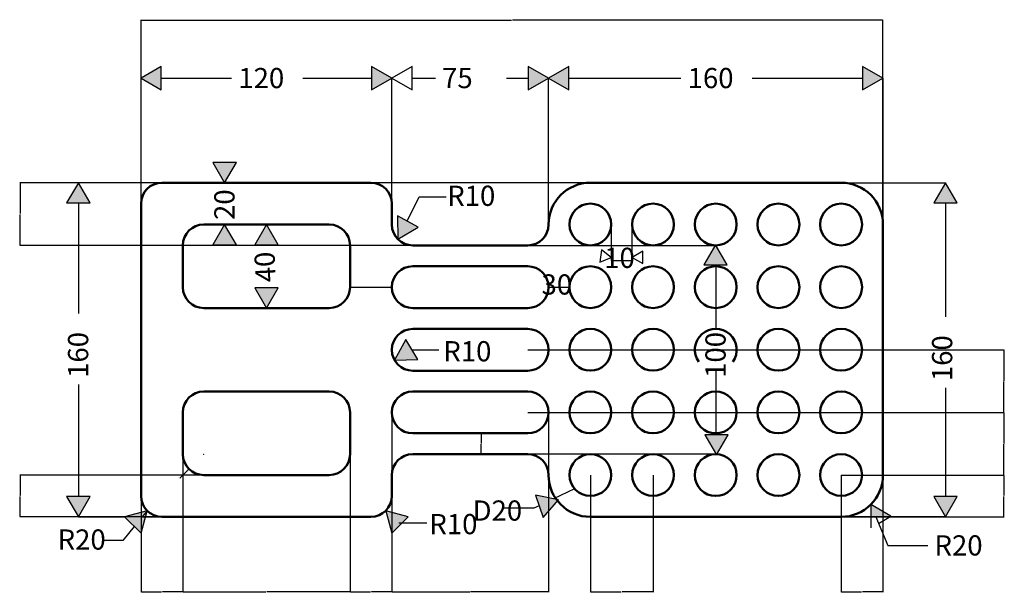
# Model space of a CAD drawing. Units: millimetres. Extents: x 384 to 855, y 1163 to 1437.
import ezdxf

# ---------------------------------------------------------------- set-up
doc = ezdxf.new("R2010")
doc.units = ezdxf.units.MM
for name, color, linetype, lineweight in [('M-DIMS', 2, 'Continuous', 25), ('M-HATC', 8, 'Continuous', 18), ('M-OUTL', 7, 'Continuous', 50), ('M-TEXT', 7, 'Continuous', 25)]:
    doc.layers.add(name, color=color, linetype=linetype, lineweight=lineweight)
doc.styles.get("Standard").update_dxf_attribs({"font": 'arial.ttf'})
doc.dimstyles.get("Standard").update_dxf_attribs({"dimtxt": 0.18, "dimasz": 0.18, "dimexe": 0.18, "dimexo": 0.0625, "dimgap": 0.09, "dimtad": 0, "dimtih": 1, "dimtoh": 1, "dimdec": 4, "dimzin": 0, "dimdsep": 46, "dimtxsty": 'Standard', "dimcen": 0.09, "dimadec": 0, "dimazin": 0, "dimtfac": 1, "dimtdec": 4, "dimtofl": 0, "dimtmove": 0, "dimatfit": 3, "dimfxl": 1, "dimtolj": 1, "dimtzin": 0, "dimarcsym": 0})

# ---------------------------------------------------------------- blocks, each defined once
blk = doc.blocks.new('HOLE-D20')
blk.add_circle((10, 10), 10)
blk = doc.blocks.new('OPENING-80X40-R10')
for p, q in [((10, 40), (70, 40)), ((0, 30), (0, 10)), ((80, 30), (80, 10)), ((10, 0), (70, 0))]:
    blk.add_line(p, q)
for centre, start, end in [((10, 30), 90, 180), ((70, 30), 0, 90), ((10, 10), 180, 270), ((70, 10), 270, 0)]:
    blk.add_arc(centre, 10, start, end)
blk = doc.blocks.new('SLOT-75X20-R10')
for p, q in [((10, 20), (65, 20)), ((10, 0), (65, 0))]:
    blk.add_line(p, q)
for centre, start, end in [((10, 10), 90, 270), ((65, 10), 270, 90)]:
    blk.add_arc(centre, 10, start, end)
blk = doc.blocks.new('DIM-ARROW-SMALL')
blk.add_lwpolyline([(0, 2.97), (5.15, 0), (5.15, 5.95)], close=True)
blk = doc.blocks.new('*D5')
at = {"layer": 'Defpoints', "color": 0, "transparency": 16777216}
for p in [(796.88, 1437.22), (441.88, 1349.32), (796.88, 1339.32)]:
    blk.add_point(p, dxfattribs=at)
at = {"layer": 'M-DIMS', "color": 0, "lineweight": -2, "transparency": 16777216}
for p, q in [((441.88, 1349.39), (441.88, 1437.4)), ((442.06, 1437.22), (619.09, 1437.22)), ((796.7, 1437.22), (619.67, 1437.22)), ((796.88, 1339.39), (796.88, 1437.4))]:
    blk.add_line(p, q, dxfattribs=at)
at = {"layer": 'M-DIMS', "color": 0, "transparency": 16777216}
for points in [[(442.06, 1437.25), (442.06, 1437.19), (441.88, 1437.22)], [(796.7, 1437.25), (796.7, 1437.19), (796.88, 1437.22)]]:
    blk.add_solid(points, dxfattribs=at)
at = {"layer": 'M-DIMS', "color": 0, "transparency": 16777216, "insert": (619.38, 1437.22), "char_height": 0.18, "attachment_point": 5}
blk.add_mtext('\\A1;355', dxfattribs=at)
blk = doc.blocks.new('*D6')
at = {"layer": 'Defpoints', "color": 0, "transparency": 16777216}
for p in [(461.88, 1229.32), (441.88, 1209.32), (461.88, 1163.36)]:
    blk.add_point(p, dxfattribs=at)
at = {"layer": 'M-DIMS', "color": 0, "lineweight": -2, "transparency": 16777216}
for p, q in [((461.88, 1229.26), (461.88, 1163.18)), ((441.88, 1209.26), (441.88, 1163.18)), ((442.06, 1163.36), (451.66, 1163.36)), ((461.7, 1163.36), (452.1, 1163.36))]:
    blk.add_line(p, q, dxfattribs=at)
at = {"layer": 'M-DIMS', "color": 0, "transparency": 16777216}
for points in [[(442.06, 1163.39), (442.06, 1163.33), (441.88, 1163.36)], [(461.7, 1163.39), (461.7, 1163.33), (461.88, 1163.36)]]:
    blk.add_solid(points, dxfattribs=at)
at = {"layer": 'M-DIMS', "color": 0, "transparency": 16777216, "insert": (451.88, 1163.36), "char_height": 0.18, "attachment_point": 5}
blk.add_mtext('\\A1;20', dxfattribs=at)
blk = doc.blocks.new('*D7')
at = {"layer": 'Defpoints', "color": 0, "transparency": 16777216}
for p in [(461.88, 1229.32), (541.88, 1229.32), (541.88, 1163.36)]:
    blk.add_point(p, dxfattribs=at)
at = {"layer": 'M-DIMS', "color": 0, "lineweight": -2, "transparency": 16777216}
for p, q in [((461.88, 1229.26), (461.88, 1163.18)), ((541.88, 1229.26), (541.88, 1163.18)), ((462.06, 1163.36), (501.66, 1163.36)), ((541.7, 1163.36), (502.1, 1163.36))]:
    blk.add_line(p, q, dxfattribs=at)
at = {"layer": 'M-DIMS', "color": 0, "transparency": 16777216}
for points in [[(462.06, 1163.39), (462.06, 1163.33), (461.88, 1163.36)], [(541.7, 1163.39), (541.7, 1163.33), (541.88, 1163.36)]]:
    blk.add_solid(points, dxfattribs=at)
at = {"layer": 'M-DIMS', "color": 0, "transparency": 16777216, "insert": (501.88, 1163.36), "char_height": 0.18, "attachment_point": 5}
blk.add_mtext('\\A1;80', dxfattribs=at)
blk = doc.blocks.new('*D8')
at = {"layer": 'Defpoints', "color": 0, "transparency": 16777216}
for p in [(561.88, 1249.32), (541.88, 1229.32), (561.88, 1163.36)]:
    blk.add_point(p, dxfattribs=at)
at = {"layer": 'M-DIMS', "color": 0, "lineweight": -2, "transparency": 16777216}
for p, q in [((561.88, 1249.26), (561.88, 1163.18)), ((541.88, 1229.26), (541.88, 1163.18)), ((542.06, 1163.36), (551.66, 1163.36)), ((561.7, 1163.36), (552.1, 1163.36))]:
    blk.add_line(p, q, dxfattribs=at)
at = {"layer": 'M-DIMS', "color": 0, "transparency": 16777216}
for points in [[(542.06, 1163.39), (542.06, 1163.33), (541.88, 1163.36)], [(561.7, 1163.39), (561.7, 1163.33), (561.88, 1163.36)]]:
    blk.add_solid(points, dxfattribs=at)
at = {"layer": 'M-DIMS', "color": 0, "transparency": 16777216, "insert": (551.88, 1163.36), "char_height": 0.18, "attachment_point": 5}
blk.add_mtext('\\A1;20', dxfattribs=at)
blk = doc.blocks.new('*D9')
at = {"layer": 'Defpoints', "color": 0, "transparency": 16777216}
for p in [(561.88, 1249.32), (636.88, 1249.32), (636.88, 1163.36)]:
    blk.add_point(p, dxfattribs=at)
at = {"layer": 'M-DIMS', "color": 0, "lineweight": -2, "transparency": 16777216}
for p, q in [((561.88, 1249.26), (561.88, 1163.18)), ((636.88, 1249.26), (636.88, 1163.18)), ((562.06, 1163.36), (599.16, 1163.36)), ((636.7, 1163.36), (599.6, 1163.36))]:
    blk.add_line(p, q, dxfattribs=at)
at = {"layer": 'M-DIMS', "color": 0, "transparency": 16777216}
for points in [[(562.06, 1163.39), (562.06, 1163.33), (561.88, 1163.36)], [(636.7, 1163.39), (636.7, 1163.33), (636.88, 1163.36)]]:
    blk.add_solid(points, dxfattribs=at)
at = {"layer": 'M-DIMS', "color": 0, "transparency": 16777216, "insert": (599.38, 1163.36), "char_height": 0.18, "attachment_point": 5}
blk.add_mtext('\\A1;75', dxfattribs=at)
blk = doc.blocks.new('*D10')
at = {"layer": 'Defpoints', "color": 0, "transparency": 16777216}
for p in [(383.98, 1219.32), (471.88, 1219.32), (451.88, 1199.32)]:
    blk.add_point(p, dxfattribs=at)
at = {"layer": 'M-DIMS', "color": 0, "lineweight": -2, "transparency": 16777216}
for p, q in [((471.82, 1219.32), (383.8, 1219.32)), ((383.98, 1219.14), (383.98, 1209.51)), ((383.98, 1199.5), (383.98, 1209.14)), ((451.82, 1199.32), (383.8, 1199.32))]:
    blk.add_line(p, q, dxfattribs=at)
at = {"layer": 'M-DIMS', "color": 0, "transparency": 16777216}
for points in [[(383.95, 1219.14), (384.01, 1219.14), (383.98, 1219.32)], [(383.95, 1199.5), (384.01, 1199.5), (383.98, 1199.32)]]:
    blk.add_solid(points, dxfattribs=at)
at = {"layer": 'M-DIMS', "color": 0, "transparency": 16777216, "insert": (383.98, 1209.32), "char_height": 0.18, "attachment_point": 5}
blk.add_mtext('\\A1;20', dxfattribs=at)
blk = doc.blocks.new('*D11')
at = {"layer": 'Defpoints', "color": 0, "transparency": 16777216}
for p in [(383.98, 1359.32), (656.88, 1359.32), (626.88, 1329.32)]:
    blk.add_point(p, dxfattribs=at)
at = {"layer": 'M-DIMS', "color": 0, "lineweight": -2, "transparency": 16777216}
for p, q in [((656.82, 1359.32), (383.8, 1359.32)), ((383.98, 1359.14), (383.98, 1344.51)), ((383.98, 1329.5), (383.98, 1344.14)), ((626.82, 1329.32), (383.8, 1329.32))]:
    blk.add_line(p, q, dxfattribs=at)
at = {"layer": 'M-DIMS', "color": 0, "transparency": 16777216}
for points in [[(383.95, 1359.14), (384.01, 1359.14), (383.98, 1359.32)], [(383.95, 1329.5), (384.01, 1329.5), (383.98, 1329.32)]]:
    blk.add_solid(points, dxfattribs=at)
at = {"layer": 'M-DIMS', "color": 0, "transparency": 16777216, "insert": (383.98, 1344.32), "char_height": 0.18, "attachment_point": 5}
blk.add_mtext('\\A1;30', dxfattribs=at)
blk = doc.blocks.new('*D12')
at = {"layer": 'Defpoints', "color": 0, "transparency": 16777216}
for p in [(626.88, 1279.32), (854.78, 1279.32), (626.88, 1249.32)]:
    blk.add_point(p, dxfattribs=at)
at = {"layer": 'M-DIMS', "color": 0, "lineweight": -2, "transparency": 16777216}
for p, q in [((626.94, 1279.32), (854.96, 1279.32)), ((854.78, 1279.14), (854.78, 1264.51)), ((854.78, 1249.5), (854.78, 1264.14)), ((626.94, 1249.32), (854.96, 1249.32))]:
    blk.add_line(p, q, dxfattribs=at)
at = {"layer": 'M-DIMS', "color": 0, "transparency": 16777216}
for points in [[(854.75, 1279.14), (854.81, 1279.14), (854.78, 1279.32)], [(854.75, 1249.5), (854.81, 1249.5), (854.78, 1249.32)]]:
    blk.add_solid(points, dxfattribs=at)
at = {"layer": 'M-DIMS', "color": 0, "transparency": 16777216, "insert": (854.78, 1264.32), "char_height": 0.18, "attachment_point": 5}
blk.add_mtext('\\A1;30', dxfattribs=at)
blk = doc.blocks.new('*D13')
at = {"layer": 'Defpoints', "color": 0, "transparency": 16777216}
for p in [(604.58, 1239.32), (626.88, 1239.32), (626.88, 1229.32)]:
    blk.add_point(p, dxfattribs=at)
at = {"layer": 'M-DIMS', "color": 0, "lineweight": -2, "transparency": 16777216}
for p, q in [((626.82, 1239.32), (604.4, 1239.32)), ((604.58, 1239.14), (604.58, 1234.51)), ((604.58, 1229.5), (604.58, 1234.14)), ((626.82, 1229.32), (604.4, 1229.32))]:
    blk.add_line(p, q, dxfattribs=at)
at = {"layer": 'M-DIMS', "color": 0, "transparency": 16777216}
for points in [[(604.55, 1239.14), (604.61, 1239.14), (604.58, 1239.32)], [(604.55, 1229.5), (604.61, 1229.5), (604.58, 1229.32)]]:
    blk.add_solid(points, dxfattribs=at)
at = {"layer": 'M-DIMS', "color": 0, "transparency": 16777216, "insert": (604.58, 1234.32), "char_height": 0.18, "attachment_point": 5}
blk.add_mtext('\\A1;10', dxfattribs=at)
blk = doc.blocks.new('*D14')
at = {"layer": 'Defpoints', "color": 0, "transparency": 16777216}
for p in [(656.88, 1219.32), (686.88, 1219.32), (686.88, 1163.36)]:
    blk.add_point(p, dxfattribs=at)
at = {"layer": 'M-DIMS', "color": 0, "lineweight": -2, "transparency": 16777216}
for p, q in [((656.88, 1219.26), (656.88, 1163.18)), ((686.88, 1219.26), (686.88, 1163.18)), ((657.06, 1163.36), (671.66, 1163.36)), ((686.7, 1163.36), (672.1, 1163.36))]:
    blk.add_line(p, q, dxfattribs=at)
at = {"layer": 'M-DIMS', "color": 0, "transparency": 16777216}
for points in [[(657.06, 1163.39), (657.06, 1163.33), (656.88, 1163.36)], [(686.7, 1163.39), (686.7, 1163.33), (686.88, 1163.36)]]:
    blk.add_solid(points, dxfattribs=at)
at = {"layer": 'M-DIMS', "color": 0, "transparency": 16777216, "insert": (671.88, 1163.36), "char_height": 0.18, "attachment_point": 5}
blk.add_mtext('\\A1;30', dxfattribs=at)
blk = doc.blocks.new('*D15')
at = {"layer": 'Defpoints', "color": 0, "transparency": 16777216}
for p in [(776.88, 1249.32), (854.78, 1249.32), (776.88, 1219.32)]:
    blk.add_point(p, dxfattribs=at)
at = {"layer": 'M-DIMS', "color": 0, "lineweight": -2, "transparency": 16777216}
for p, q in [((776.94, 1249.32), (854.96, 1249.32)), ((854.78, 1249.14), (854.78, 1234.51)), ((854.78, 1219.5), (854.78, 1234.14)), ((776.94, 1219.32), (854.96, 1219.32))]:
    blk.add_line(p, q, dxfattribs=at)
at = {"layer": 'M-DIMS', "color": 0, "transparency": 16777216}
for points in [[(854.75, 1249.14), (854.81, 1249.14), (854.78, 1249.32)], [(854.75, 1219.5), (854.81, 1219.5), (854.78, 1219.32)]]:
    blk.add_solid(points, dxfattribs=at)
at = {"layer": 'M-DIMS', "color": 0, "transparency": 16777216, "insert": (854.78, 1234.32), "char_height": 0.18, "attachment_point": 5}
blk.add_mtext('\\A1;30', dxfattribs=at)
blk = doc.blocks.new('*D16')
at = {"layer": 'Defpoints', "color": 0, "transparency": 16777216}
for p in [(776.88, 1219.32), (796.88, 1219.32), (796.88, 1163.36)]:
    blk.add_point(p, dxfattribs=at)
at = {"layer": 'M-DIMS', "color": 0, "lineweight": -2, "transparency": 16777216}
for p, q in [((776.88, 1219.26), (776.88, 1163.18)), ((796.88, 1219.26), (796.88, 1163.18)), ((777.06, 1163.36), (786.66, 1163.36)), ((796.7, 1163.36), (787.1, 1163.36))]:
    blk.add_line(p, q, dxfattribs=at)
at = {"layer": 'M-DIMS', "color": 0, "transparency": 16777216}
for points in [[(777.06, 1163.39), (777.06, 1163.33), (776.88, 1163.36)], [(796.7, 1163.39), (796.7, 1163.33), (796.88, 1163.36)]]:
    blk.add_solid(points, dxfattribs=at)
at = {"layer": 'M-DIMS', "color": 0, "transparency": 16777216, "insert": (786.88, 1163.36), "char_height": 0.18, "attachment_point": 5}
blk.add_mtext('\\A1;20', dxfattribs=at)
blk = doc.blocks.new('*D17')
at = {"layer": 'Defpoints', "color": 0, "transparency": 16777216}
for p in [(776.88, 1219.32), (854.78, 1219.32), (776.88, 1199.32)]:
    blk.add_point(p, dxfattribs=at)
at = {"layer": 'M-DIMS', "color": 0, "lineweight": -2, "transparency": 16777216}
for p, q in [((776.94, 1219.32), (854.96, 1219.32)), ((854.78, 1219.14), (854.78, 1209.51)), ((854.78, 1199.5), (854.78, 1209.14)), ((776.94, 1199.32), (854.96, 1199.32))]:
    blk.add_line(p, q, dxfattribs=at)
at = {"layer": 'M-DIMS', "color": 0, "transparency": 16777216}
for points in [[(854.75, 1219.14), (854.81, 1219.14), (854.78, 1219.32)], [(854.75, 1199.5), (854.81, 1199.5), (854.78, 1199.32)]]:
    blk.add_solid(points, dxfattribs=at)
at = {"layer": 'M-DIMS', "color": 0, "transparency": 16777216, "insert": (854.78, 1209.32), "char_height": 0.18, "attachment_point": 5}
blk.add_mtext('\\A1;20', dxfattribs=at)
blk = doc.blocks.new('*D18')
at = {"layer": 'Defpoints', "color": 0, "transparency": 16777216}
for p in [(471.88, 1229.32), (464.81, 1222.25)]:
    blk.add_point(p, dxfattribs=at)
at = {"layer": 'M-DIMS', "color": 0, "lineweight": -2, "transparency": 16777216}
for p, q in [((471.79, 1229.32), (471.97, 1229.32)), ((471.88, 1229.23), (471.88, 1229.41)), ((460.57, 1218.01), (464.68, 1222.12)), ((460.39, 1218.01), (460.57, 1218.01))]:
    blk.add_line(p, q, dxfattribs=at)
at = {"layer": 'M-DIMS', "color": 0, "transparency": 16777216}
blk.add_solid([(464.66, 1222.15), (464.71, 1222.1), (464.81, 1222.25)], dxfattribs=at)
at = {"layer": 'M-DIMS', "color": 0, "transparency": 16777216, "insert": (459.89, 1218.01), "char_height": 0.18, "attachment_point": 5}
blk.add_mtext('\\A1;8X R10', dxfattribs=at)

msp = doc.modelspace()

# ---------------------------------------------------------------- hatches: boundary and pattern name
at = {"layer": 'M-HATC'}
h = msp.add_hatch(color=256, dxfattribs=at)
h.dxf.hatch_style = 1
h.paths.add_polyline_path([(411.88, 1359.32), (406.28, 1349.63), (417.48, 1349.63)])
h.paths.add_polyline_path([(417.48, 1209.02), (406.28, 1209.02), (411.88, 1199.32)])
h.paths.add_polyline_path([(444.03, 1199.32), (442.41, 1199.32), (444.81, 1202.25), (434, 1199.36), (441.91, 1191.44)])
h.paths.add_polyline_path([(487.48, 1369.02), (476.28, 1369.02), (481.88, 1359.32)])
h.paths.add_polyline_path([(481.88, 1339.32), (476.28, 1329.63), (487.48, 1329.63)])
h.paths.add_polyline_path([(501.88, 1339.32), (496.28, 1329.63), (507.48, 1329.63)])
h.paths.add_polyline_path([(507.48, 1309.02), (496.28, 1309.02), (501.88, 1299.32)])
h.paths.add_polyline_path([(451.58, 1414.92), (441.88, 1409.32), (451.58, 1403.73)])
h.paths.add_polyline_path([(552.18, 1414.92), (552.18, 1403.73), (561.88, 1409.32)])
h.paths.add_polyline_path([(574.42, 1338.01), (564.63, 1343.45), (564.81, 1332.25)])
h.paths.add_polyline_path([(636.88, 1409.32), (627.18, 1414.92), (627.18, 1403.73)])
h.paths.add_polyline_path([(646.58, 1414.92), (636.88, 1409.32), (646.58, 1403.73)])
h.paths.add_polyline_path([(787.18, 1414.92), (787.18, 1403.73), (796.88, 1409.32)])
h.paths.add_polyline_path([(826.88, 1359.32), (821.28, 1349.63), (832.48, 1349.63)])
h.paths.add_polyline_path([(832.48, 1209.02), (821.28, 1209.02), (826.88, 1199.32)])
h.paths.add_polyline_path([(791.02, 1205.18), (791.02, 1199.32), (800.27, 1199.32), (800.72, 1199.58)])
h.paths.add_polyline_path([(641.17, 1206.95, -0.012246), (640.58, 1207.73), (630.67, 1209.63), (634.35, 1199.05)])
h.paths.add_polyline_path([(558.95, 1202.25), (561.85, 1191.44), (569.77, 1199.36)])
h.paths.add_polyline_path([(568.51, 1284.25), (563.17, 1274.41), (574.36, 1274.71)])
h.paths.add_polyline_path([(716.98, 1329.32), (716.6, 1329.32), (711.19, 1319.96), (722.39, 1319.96)])
h.paths.add_polyline_path([(726.88, 1219.32, -1), (706.88, 1219.32, -0.414214), (716.88, 1229.32), (716.88, 1229.59), (711.64, 1238.66), (716.88, 1238.66), (716.88, 1239.32, -0.414214), (706.88, 1249.32, -1), (726.88, 1249.32, -0.414214), (716.88, 1239.32), (716.88, 1238.66), (722.84, 1238.66), (717.44, 1229.31, -0.397898)])
h.paths.add_polyline_path([(726.88, 1219.32, 0.397898), (717.44, 1229.31), (717.24, 1228.96), (717.03, 1229.32, 0.418706), (706.88, 1219.32, 1)])
h.paths.add_polyline_path([(716.88, 1259.32, 0.414214), (706.88, 1249.32, 0.414214), (716.88, 1239.32)], flags=17)
h.paths.add_polyline_path([(716.88, 1259.32), (716.88, 1239.32, 0.414214), (726.88, 1249.32, 0.414214)], flags=17)

# ---------------------------------------------------------------- linework, layer by layer
at = {"layer": 'M-DIMS'}
for p, q in [((441.88, 1349.32), (441.88, 1409.32)), ((451.58, 1409.32), (485.21, 1409.32)), ((519.27, 1409.32), (552.18, 1409.32)), ((561.88, 1339.32), (561.88, 1409.32)), ((571.58, 1409.32), (582.71, 1409.32)), ((616.77, 1409.32), (627.18, 1409.32)), ((636.88, 1339.32), (636.88, 1409.32)), ((646.58, 1409.32), (700.21, 1409.32)), ((734.27, 1409.32), (787.18, 1409.32)), ((796.88, 1409.32), (796.88, 1339.32)), ((451.88, 1359.32), (411.88, 1359.32)), ((501.88, 1359.32), (461.88, 1359.32)), ((776.88, 1359.32), (796.88, 1359.32)), ((796.88, 1359.32), (826.88, 1359.32)), ((569.15, 1340.93), (574.95, 1352.5)), ((574.95, 1352.5), (587.94, 1352.5)), ((411.88, 1349.63), (411.88, 1296.71)), ((826.88, 1349.63), (826.88, 1295.15)), ((666.88, 1339.32), (666.88, 1322.08)), ((676.88, 1322.08), (676.88, 1339.32)), ((626.88, 1329.32), (716.88, 1329.32)), ((666.88, 1322.08), (676.88, 1322.08)), ((716.88, 1319.96), (716.88, 1289.32)), ((541.88, 1309.32), (561.88, 1309.32)), ((636.88, 1309.32), (646.88, 1309.32)), ((571.62, 1279.18), (571.88, 1279.32)), ((571.88, 1279.32), (584.29, 1279.32)), ((716.88, 1269.32), (716.88, 1238.66)), ((411.88, 1262.66), (411.88, 1209.02)), ((826.88, 1261.1), (826.88, 1209.02)), ((716.88, 1229.32), (626.88, 1229.32)), ((716.88, 1229.59), (716.88, 1229.32)), ((649.32, 1212.78), (639.31, 1207.97)), ((444.81, 1202.25), (442.41, 1199.32)), ((629.79, 1203.41), (615.58, 1203.41)), ((632.4, 1204.66), (629.79, 1203.41)), ((411.88, 1199.32), (434.03, 1199.32)), ((442.41, 1199.32), (451.88, 1199.32)), ((826.88, 1199.32), (776.88, 1199.32)), ((793.49, 1199.32), (799.23, 1185.66)), ((438.63, 1194.72), (433.12, 1188.01)), ((565.2, 1196.51), (578.6, 1196.51)), ((433.12, 1188.01), (423.38, 1188.01)), ((799.23, 1185.66), (818.32, 1185.66))]:
    msp.add_line(p, q, dxfattribs=at)
for points in [[(441.88, 1409.32), (451.58, 1403.73), (451.58, 1414.92)], [(561.88, 1409.32), (552.18, 1414.92), (552.18, 1403.73)], [(561.88, 1409.32), (571.58, 1403.73), (571.58, 1414.92)], [(636.88, 1409.32), (627.18, 1414.92), (627.18, 1403.73)], [(636.88, 1409.32), (646.58, 1403.73), (646.58, 1414.92)], [(796.88, 1409.32), (787.18, 1414.92), (787.18, 1403.73)], [(481.88, 1359.32), (487.48, 1369.02), (476.28, 1369.02)], [(411.88, 1359.32), (406.28, 1349.63), (417.48, 1349.63)], [(826.88, 1359.32), (821.28, 1349.63), (832.48, 1349.63)], [(564.63, 1343.45), (564.81, 1332.25), (574.42, 1338.01)], [(481.88, 1339.32), (476.28, 1329.63), (487.48, 1329.63)], [(501.88, 1339.32), (496.28, 1329.63), (507.48, 1329.63)], [(716.79, 1329.66), (711.19, 1319.96), (722.39, 1319.96)], [(501.88, 1299.32), (507.48, 1309.02), (496.28, 1309.02)], [(568.51, 1284.25), (563.17, 1274.41), (574.36, 1274.71)], [(717.24, 1228.96), (722.84, 1238.66), (711.64, 1238.66)], [(411.88, 1199.32), (417.48, 1209.02), (406.28, 1209.02)], [(630.67, 1209.63), (634.35, 1199.05), (641.67, 1207.52)], [(826.88, 1199.32), (832.48, 1209.02), (821.28, 1209.02)], [(444.81, 1202.25), (434, 1199.36), (441.91, 1191.44)], [(558.95, 1202.25), (561.85, 1191.44), (569.77, 1199.36)]]:
    msp.add_lwpolyline(points, close=True, dxfattribs=at)
msp.add_lwpolyline([(794.81, 1196.17), (800.72, 1199.58), (791.02, 1205.18), (791.02, 1193.99)], dxfattribs=at)
at = {"layer": 'M-OUTL'}
for p, q in [((551.88, 1359.32), (451.88, 1359.32)), ((656.88, 1359.32), (776.88, 1359.32)), ((441.88, 1209.32), (441.88, 1349.32)), ((561.88, 1339.32), (561.88, 1349.32)), ((796.88, 1339.32), (796.88, 1219.32)), ((571.88, 1329.32), (626.88, 1329.32)), ((571.88, 1229.32), (626.88, 1229.32)), ((561.88, 1209.32), (561.88, 1219.32)), ((451.88, 1199.32), (551.88, 1199.32)), ((656.88, 1199.32), (776.88, 1199.32))]:
    msp.add_line(p, q, dxfattribs=at)
for centre in [(716.88, 1249.32), (716.88, 1219.32)]:
    msp.add_circle(centre, 10, dxfattribs=at)
for centre, radius, start, end in [((451.88, 1349.32), 10, 90, 180), ((551.88, 1349.32), 10, 0, 90), ((656.88, 1339.32), 20, 90, 180), ((776.88, 1339.32), 20, 0, 90), ((571.88, 1339.32), 10, 180, 270), ((626.88, 1339.32), 10, 270, 0), ((716.88, 1279.32), 10, 324.5283, 215.1776), ((571.88, 1219.32), 10, 90, 180), ((626.88, 1219.32), 10, 0, 90), ((656.88, 1219.32), 20, 180, 270), ((776.88, 1219.32), 20, 270, 0), ((451.88, 1209.32), 10, 180, 270), ((551.88, 1209.32), 10, 270, 0)]:
    msp.add_arc(centre, radius, start, end, dxfattribs=at)

# ---------------------------------------------------------------- block references
at = {"layer": 'M-DIMS', "rotation": 171.8056456691831}
msp.add_blockref('DIM-ARROW-SMALL', (667.31, 1326.51), dxfattribs=at)
at = {"layer": 'M-DIMS'}
msp.add_blockref('DIM-ARROW-SMALL', (676.88, 1320.59), dxfattribs=at)
at = {"layer": 'M-OUTL'}
for name, p in [('HOLE-D20', (646.88, 1329.33)), ('HOLE-D20', (676.88, 1329.33)), ('HOLE-D20', (706.88, 1329.33)), ('HOLE-D20', (736.88, 1329.33)), ('HOLE-D20', (766.88, 1329.33)), ('OPENING-80X40-R10', (461.88, 1299.33)), ('SLOT-75X20-R10', (561.88, 1299.33)), ('HOLE-D20', (646.88, 1299.33)), ('HOLE-D20', (676.88, 1299.33)), ('HOLE-D20', (706.88, 1299.33)), ('HOLE-D20', (736.88, 1299.33)), ('HOLE-D20', (766.88, 1299.33)), ('HOLE-D20', (646.88, 1269.33)), ('HOLE-D20', (676.88, 1269.33)), ('HOLE-D20', (736.88, 1269.33)), ('HOLE-D20', (766.88, 1269.33)), ('OPENING-80X40-R10', (461.88, 1219.33)), ('HOLE-D20', (646.88, 1239.33)), ('HOLE-D20', (676.88, 1239.33)), ('HOLE-D20', (736.88, 1239.33)), ('HOLE-D20', (766.88, 1239.33)), ('HOLE-D20', (646.88, 1209.33)), ('HOLE-D20', (676.88, 1209.33)), ('HOLE-D20', (736.88, 1209.33)), ('HOLE-D20', (766.88, 1209.33))]:
    msp.add_blockref(name, p, dxfattribs=at)
at = {"layer": 'M-OUTL', "rotation": 180}
for p in [(636.88, 1289.32), (636.88, 1259.32)]:
    msp.add_blockref('SLOT-75X20-R10', p, dxfattribs=at)

# ---------------------------------------------------------------- texts
at = {"layer": 'M-TEXT', "char_height": 9.668, "attachment_point": 1}
for s, insert in [('120', (488.43, 1414.28)), ('75', (585.93, 1414.28)), ('160', (703.43, 1414.28)), ('R10', (588.37, 1357.9)), ('10', (663.51, 1328.19)), ('30', (633.51, 1315.43)), ('R10', (586.5, 1283.46)), ('D20', (600.53, 1207.18)), ('R10', (579.83, 1200.69)), ('R20', (401.95, 1193.3)), ('R20', (821.55, 1190.48))]:
    msp.add_mtext_dynamic_manual_height_columns(s, width=27.6087, gutter_width=48.34, heights=[0], dxfattribs=dict(at, insert=insert))
for s, insert, rotation in [('20', (476.93, 1341.5), 90), ('40', (496.79, 1311.41), 92.964), ('160', (406.93, 1265.88), 90), ('100', (711.93, 1265.88), 90), ('160', (820.37, 1264.32), 90)]:
    msp.add_mtext_dynamic_manual_height_columns(s, width=27.6087, gutter_width=48.34, heights=[0], dxfattribs=dict(at, insert=insert, rotation=rotation))

# ---------------------------------------------------------------- dimensions: what is measured, and where the dimension line sits
at = {"layer": 'M-DIMS'}
for base, p1, p2, picture, middle in [((796.88, 1437.22), (441.88, 1349.32), (796.88, 1339.32), '*D5', (619.38, 1437.22)), ((561.88, 1163.36), (541.88, 1229.32), (561.88, 1249.32), '*D8', (551.88, 1163.36)), ((636.88, 1163.36), (561.88, 1249.32), (636.88, 1249.32), '*D9', (599.38, 1163.36)), ((461.88, 1163.36), (441.88, 1209.32), (461.88, 1229.32), '*D6', (451.88, 1163.36)), ((541.88, 1163.36), (461.88, 1229.32), (541.88, 1229.32), '*D7', (501.88, 1163.36)), ((686.88, 1163.36), (656.88, 1219.32), (686.88, 1219.32), '*D14', (671.88, 1163.36)), ((796.88, 1163.36), (776.88, 1219.32), (796.88, 1219.32), '*D16', (786.88, 1163.36))]:
    dim = msp.add_linear_dim(base=base, p1=p1, p2=p2, dimstyle='Standard', override={"dimdec": 0, "dimlfac": 1, "dimrnd": 0, "dimzin": 0, "dimdsep": 46, "dimlunit": 2}, dxfattribs=at)
    dim.commit()
    dim.dimension.update_dxf_attribs({"geometry": picture, "text_midpoint": middle})
for base, p1, p2, picture, middle in [((383.98, 1359.32), (626.88, 1329.32), (656.88, 1359.32), '*D11', (383.98, 1344.32)), ((854.78, 1279.32), (626.88, 1249.32), (626.88, 1279.32), '*D12', (854.78, 1264.32)), ((854.78, 1249.32), (776.88, 1219.32), (776.88, 1249.32), '*D15', (854.78, 1234.32)), ((604.58, 1239.32), (626.88, 1229.32), (626.88, 1239.32), '*D13', (604.58, 1234.32)), ((383.98, 1219.32), (451.88, 1199.32), (471.88, 1219.32), '*D10', (383.98, 1209.32)), ((854.78, 1219.32), (776.88, 1199.32), (776.88, 1219.32), '*D17', (854.78, 1209.32))]:
    dim = msp.add_linear_dim(base=base, p1=p1, p2=p2, angle=90, dimstyle='Standard', override={"dimdec": 0, "dimlfac": 1, "dimrnd": 0, "dimzin": 0, "dimdsep": 46, "dimlunit": 2}, dxfattribs=at)
    dim.commit()
    dim.dimension.update_dxf_attribs({"geometry": picture, "text_midpoint": middle})
dim = msp.add_radius_dim(center=(471.88, 1229.32), mpoint=(464.81, 1222.25), text='8X <>', dimstyle='Standard', override={"dimdec": 0, "dimlfac": 1, "dimrnd": 0, "dimzin": 0, "dimdsep": 46, "dimlunit": 2}, dxfattribs=at)
dim.commit()
dim.dimension.update_dxf_attribs({"geometry": '*D18', "text_midpoint": (459.89, 1218.01), "dimtype": 164})

doc.saveas('drawing.dxf')
